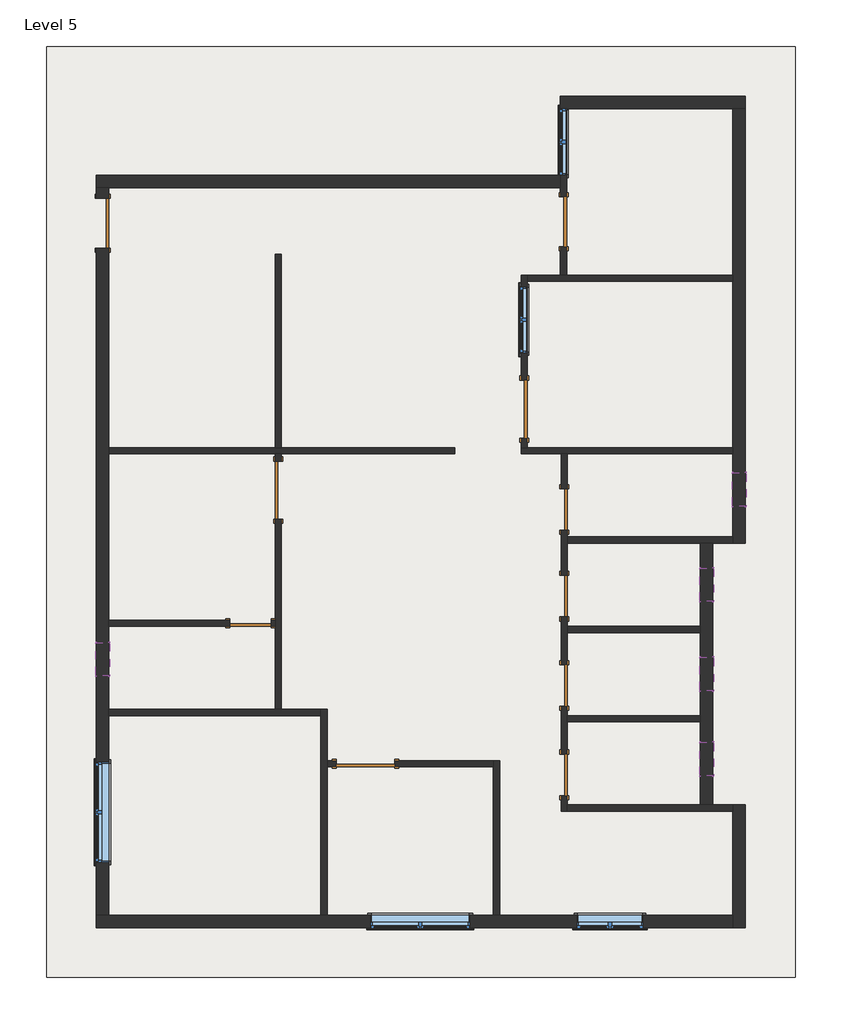
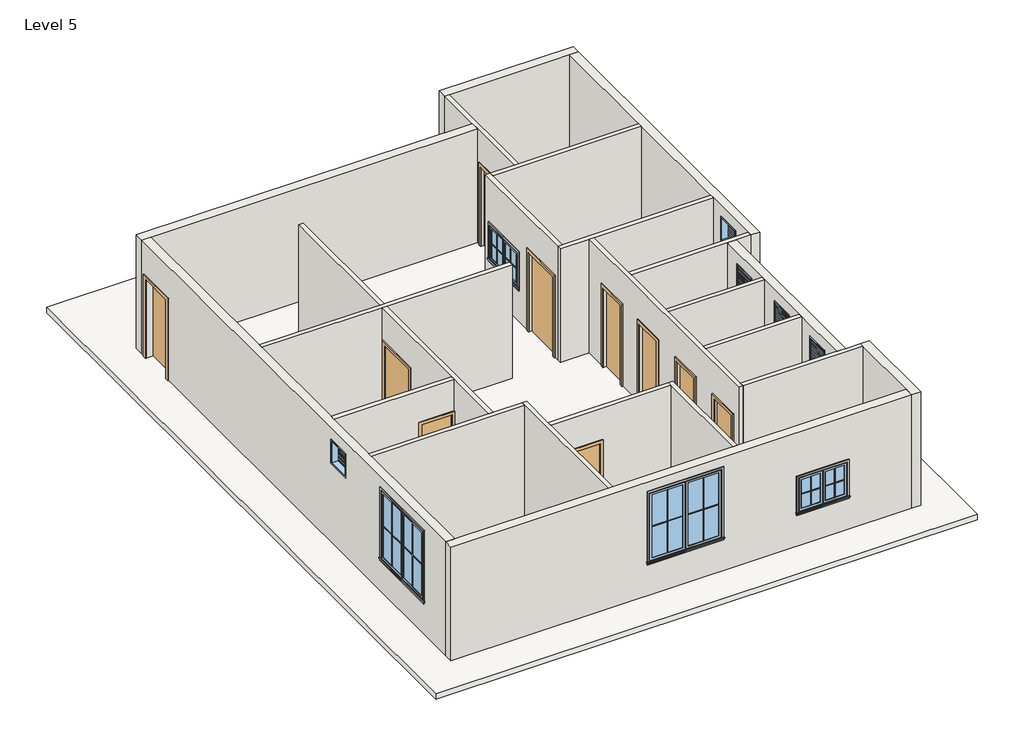
# One storey, incomplete: 23 walls, 20 proxies, 10 doors, 10 windows, 1 roof.
# Revit data of these elements (continued)
# Elements 48, 49, 50, 51, 52, 53, 54 (IfcWall, "WALL 9\"") (continued)
#   Base Offset = 0' - 0"
#   Unconnected Height = 10' - 0"
#   wall height = 10' - 0"
#   Phase Created = New Construction
#   Base Constraint = Level 5
#   Materials on its faces: "Default Wall", "Wood - Stained"
# Element 55 (IfcWindow, "Window-Casement-Double : WIN 4'")
#   Mark = "43"
#   Window Inset = 0' - 0"
#   Interior Wall Closure = 0' - 2 1/4"
#   Frame Extension = 0' - 0 1/4"
#   Exterior Wall Closure = 0' - 1 1/4"
#   Interior Trim Visibility = yes
#   Exterior Trim Visibility = yes
#   Phase Created = New Construction
#   Materials on its faces: "Wood - Stained", "Glass", "Clad - White"
# Element 56 (IfcWindow, "Window-Casement-Double : WIN 4'")
#   Mark = "44"
#   Window Inset = 0' - 0"
#   Interior Wall Closure = 0' - 2 1/4"
#   Frame Extension = 0' - 0 1/4"
#   Exterior Wall Closure = 0' - 1 1/4"
#   Interior Trim Visibility = yes
#   Exterior Trim Visibility = yes
#   Phase Created = New Construction
#   Materials on its faces: "Wood - Stained", "Glass", "Clad - White"
# Element 57 (IfcWindow, "Window-Casement-Double : WIN 4'")
#   Mark = "45"
#   Window Inset = 0' - 0"
#   Interior Wall Closure = 0' - 2 1/4"
#   Frame Extension = 0' - 0 1/4"
#   Exterior Wall Closure = 0' - 1 1/4"
#   Interior Trim Visibility = yes
#   Exterior Trim Visibility = yes
#   Phase Created = New Construction
#   Materials on its faces: "Wood - Stained", "Glass", "Clad - White"
# Element 58 (IfcWindow, "Window-Casement-Double : WIN 6'")
#   Mark = "41"
#   Window Inset = 0' - 0"
#   Interior Wall Closure = 0' - 2 1/4"
#   Frame Extension = 0' - 0 1/4"
#   Exterior Wall Closure = 0' - 1 1/4"
#   Interior Trim Visibility = yes
#   Exterior Trim Visibility = yes
#   Phase Created = New Construction
#   Materials on its faces: "Wood - Stained", "Glass", "Clad - White"
# Element 59 (IfcWindow, "Window-Casement-Double : WIN 6'")
#   Mark = "42"
#   Window Inset = 0' - 0"
#   Interior Wall Closure = 0' - 2 1/4"
#   Frame Extension = 0' - 0 1/4"
#   Exterior Wall Closure = 0' - 1 1/4"
#   Interior Trim Visibility = yes
#   Exterior Trim Visibility = yes
#   Phase Created = New Construction
#   Materials on its faces: "Wood - Stained", "Glass", "Clad - White"
# Element 60 (IfcWindow, "Window-Louvers : 24\" x 24\"")
#   Mark = "46"
#   Blade Width = 1' - 10 1/2"
#   Phase Created = New Construction
#   Materials on its faces: "Birch"
# Element 61 (IfcWindow, "Window-Louvers : 24\" x 24\"")
#   Mark = "47"
#   Blade Width = 1' - 10 1/2"
#   Phase Created = New Construction
#   Materials on its faces: "Birch"
# Element 62 (IfcWindow, "Window-Louvers : 24\" x 24\"")
#   Mark = "48"
#   Blade Width = 1' - 10 1/2"
#   Phase Created = New Construction
#   Materials on its faces: "Birch"
# Element 63 (IfcWindow, "Window-Louvers : 24\" x 24\"")
#   Mark = "49"
#   Blade Width = 1' - 10 1/2"
#   Phase Created = New Construction
#   Materials on its faces: "Birch"
# Element 64 (IfcWindow, "Window-Louvers : 24\" x 24\"")
#   Mark = "50"
#   Blade Width = 1' - 10 1/2"
#   Phase Created = New Construction
#   Materials on its faces: "Birch"
# Materials
#   "Door - Panel": class "Wood", colour RGB 210 159 95, transparency 0, Cost = 0
#   "Door - Frame": colour RGB 118 70 51, transparency 0, Cost = 0
#   "Wood - Stained": class "Wood", colour RGB 224 178 126, transparency 0, Cost = 0
#   "Glass": class "Glass", colour RGB 0 128 192, transparency 0.75, Description = "Soda Lime Glass", Cost = 0
#   "Clad - White": class "Wood", colour RGB 242 242 238, transparency 0, Cost = 0
#   "Birch": class "Wood", colour RGB 224 178 126, transparency 0, Description = "Betula Alleghaniensis", Cost = 0
#   "Default Roof": colour RGB 88 101 114, transparency 0, Cost = 0
#   "Cherry": class "Wood", colour RGB 226 177 128, transparency 0, Description = "Prunus Serotina", Cost = 0
#   "Wood Planks": class "Wood", colour RGB 193 160 115, transparency 0, Description = "Physical material.", Cost = 0
#   "Default Wall": colour RGB 128 128 128, transparency 0, Cost = 0
